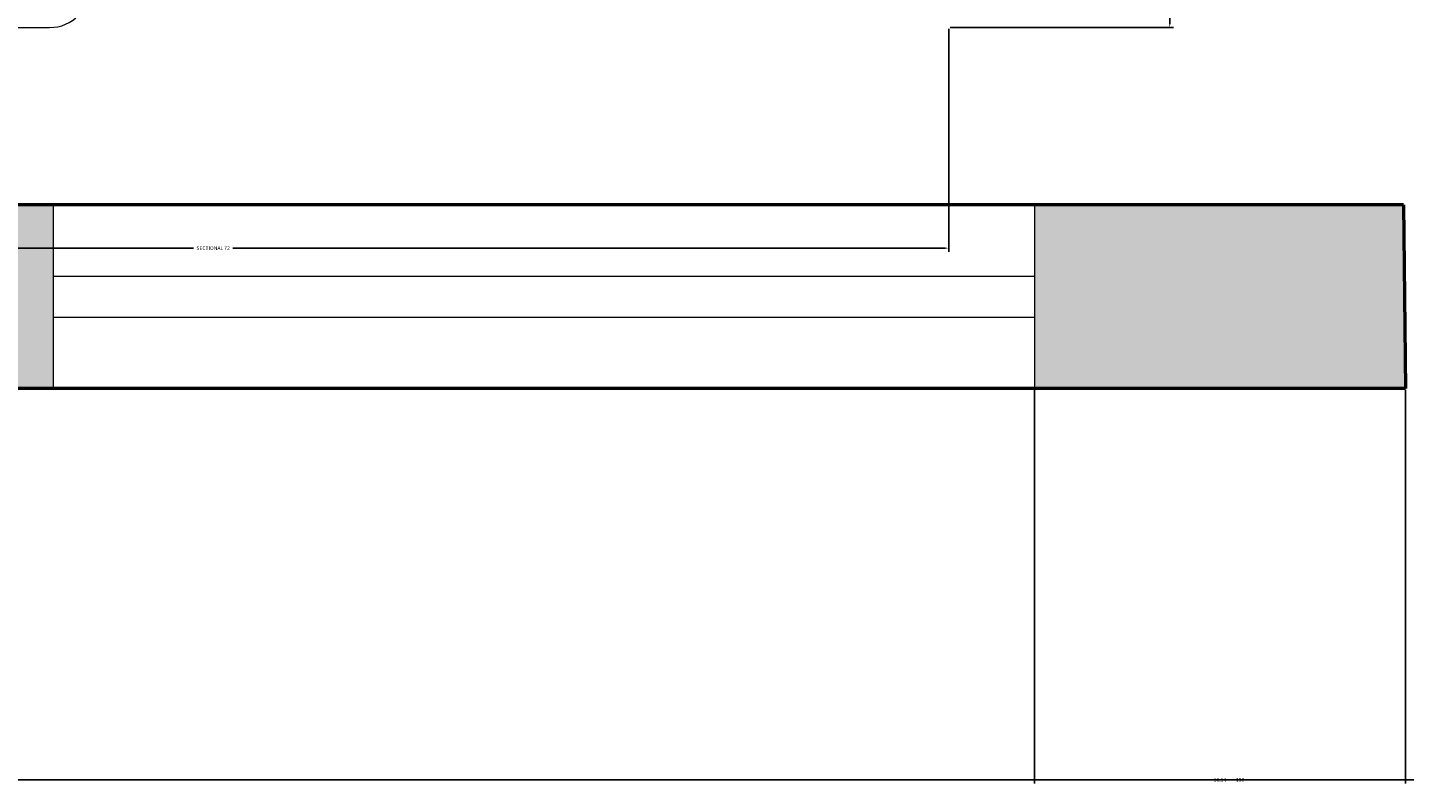
# Model space of a CAD drawing. Units: inches. Extents: x 2307 to 2544, y 2171 to 2540.
# Tile 2 of 52: x 2366 to 2434, y 2171 to 2208. Entities that reach past the tile are written whole.
import ezdxf

# ---------------------------------------------------------------- set-up
doc = ezdxf.new("R2010")
doc.units = ezdxf.units.IN
for name, color, linetype, lineweight in [('A-ANNO-DIMS', 2, 'Continuous', 18), ('A-FURN', 8, 'Continuous', 18), ('A-GLAZ', 4, 'Continuous', 18), ('A-WALL', 7, 'Continuous', 50)]:
    doc.layers.add(name, color=color, linetype=linetype, lineweight=lineweight)
doc.layers.add('A-WALL-PATT', color=18, linetype='Continuous', lineweight=13, true_color=0x000000)
doc.styles.get("Standard").update_dxf_attribs({"font": 'arial.ttf'})
doc.dimstyles.get("Standard").update_dxf_attribs({"dimtxt": 0.18, "dimasz": 0.18, "dimexe": 0.18, "dimexo": 0.0625, "dimgap": 0.09, "dimtad": 0, "dimtih": 1, "dimtoh": 1, "dimdec": 4, "dimzin": 0, "dimdsep": 46, "dimtxsty": 'Standard', "dimcen": 0.09, "dimadec": 0, "dimazin": 0, "dimtfac": 1, "dimtdec": 4, "dimtofl": 0, "dimtmove": 0, "dimatfit": 3, "dimfxl": 1, "dimtolj": 1, "dimtzin": 0, "dimarcsym": 0})

# ---------------------------------------------------------------- blocks, each defined once
blk = doc.blocks.new('sofa')
blk.add_line((-19, -66), (7, -66))
blk.add_arc((7, -64), 2, 270, 0)
blk = doc.blocks.new('WIN-48IN')
for p, q in [((0, 5.5), (48, 5.5)), ((0, 3.5), (48, 3.5))]:
    blk.add_line(p, q)
for points in [[(0, 0), (0, 9)], [(48, 9), (48, 0)]]:
    blk.add_lwpolyline(points)
blk = doc.blocks.new('*D34')
at = {"layer": 'A-ANNO-DIMS', "color": 0, "lineweight": -2, "transparency": 16777216}
for p, q in [((2339.456, 2208.123), (2339.456, 2197.206)), ((2411.456, 2208.123), (2411.456, 2197.206)), ((2339.636, 2197.386), (2374.491, 2197.386)), ((2411.276, 2197.386), (2376.421, 2197.386))]:
    blk.add_line(p, q, dxfattribs=at)
at = {"layer": 'A-ANNO-DIMS', "color": 0, "transparency": 16777216}
for points in [[(2339.636, 2197.416), (2339.636, 2197.356), (2339.456, 2197.386)], [(2411.276, 2197.416), (2411.276, 2197.356), (2411.456, 2197.386)]]:
    blk.add_solid(points, dxfattribs=at)
at = {"layer": 'Defpoints', "color": 0, "transparency": 16777216}
for p in [(2339.456, 2208.186), (2411.456, 2208.186), (2411.456, 2197.386)]:
    blk.add_point(p, dxfattribs=at)
at = {"layer": 'A-ANNO-DIMS', "color": 0, "transparency": 16777216, "insert": (2375.456, 2197.386), "char_height": 0.18, "attachment_point": 5}
blk.add_mtext('\\A1;SECTIONAL 72', dxfattribs=at)
blk = doc.blocks.new('*D35')
at = {"layer": 'A-ANNO-DIMS', "color": 0, "lineweight": -2, "transparency": 16777216}
for p, q in [((2411.518, 2280.186), (2422.436, 2280.186)), ((2422.256, 2280.006), (2422.256, 2244.366)), ((2422.256, 2208.366), (2422.256, 2244.005)), ((2411.518, 2208.186), (2422.436, 2208.186))]:
    blk.add_line(p, q, dxfattribs=at)
at = {"layer": 'A-ANNO-DIMS', "color": 0, "transparency": 16777216}
for points in [[(2422.226, 2280.006), (2422.286, 2280.006), (2422.256, 2280.186)], [(2422.226, 2208.366), (2422.286, 2208.366), (2422.256, 2208.186)]]:
    blk.add_solid(points, dxfattribs=at)
at = {"layer": 'Defpoints', "color": 0, "transparency": 16777216}
for p in [(2411.456, 2280.186), (2422.256, 2280.186), (2411.456, 2208.186)]:
    blk.add_point(p, dxfattribs=at)
at = {"layer": 'A-ANNO-DIMS', "color": 0, "transparency": 16777216, "insert": (2422.256, 2244.186), "char_height": 0.18, "attachment_point": 5}
blk.add_mtext('\\A1;72', dxfattribs=at)
blk = doc.blocks.new('*D36')
at = {"layer": 'A-ANNO-DIMS', "color": 0, "lineweight": -2, "transparency": 16777216}
for p, q in [((2326.696, 2190.447), (2326.696, 2171.18)), ((2524.696, 2190.447), (2524.696, 2171.18)), ((2326.876, 2171.36), (2425.415, 2171.36)), ((2524.516, 2171.36), (2425.976, 2171.36))]:
    blk.add_line(p, q, dxfattribs=at)
at = {"layer": 'A-ANNO-DIMS', "color": 0, "transparency": 16777216}
for points in [[(2326.876, 2171.39), (2326.876, 2171.33), (2326.696, 2171.36)], [(2524.516, 2171.39), (2524.516, 2171.33), (2524.696, 2171.36)]]:
    blk.add_solid(points, dxfattribs=at)
at = {"layer": 'Defpoints', "color": 0, "transparency": 16777216}
for p in [(2326.696, 2190.51), (2524.696, 2190.51), (2524.696, 2171.36)]:
    blk.add_point(p, dxfattribs=at)
at = {"layer": 'A-ANNO-DIMS', "color": 0, "transparency": 16777216, "insert": (2425.696, 2171.36), "char_height": 0.18, "attachment_point": 5}
blk.add_mtext('\\A1;198', dxfattribs=at)
blk = doc.blocks.new('*D38')
at = {"layer": 'A-ANNO-DIMS', "color": 0, "lineweight": -2, "transparency": 16777216}
for p, q in [((2415.642, 2190.447), (2415.642, 2171.18)), ((2433.783, 2190.447), (2433.783, 2171.18)), ((2415.822, 2171.36), (2424.328, 2171.36)), ((2433.603, 2171.36), (2425.098, 2171.36))]:
    blk.add_line(p, q, dxfattribs=at)
at = {"layer": 'A-ANNO-DIMS', "color": 0, "transparency": 16777216}
for points in [[(2415.822, 2171.39), (2415.822, 2171.33), (2415.642, 2171.36)], [(2433.603, 2171.39), (2433.603, 2171.33), (2433.783, 2171.36)]]:
    blk.add_solid(points, dxfattribs=at)
at = {"layer": 'Defpoints', "color": 0, "transparency": 16777216}
for p in [(2415.642, 2190.51), (2433.783, 2190.51), (2433.783, 2171.36)]:
    blk.add_point(p, dxfattribs=at)
at = {"layer": 'A-ANNO-DIMS', "color": 0, "transparency": 16777216, "insert": (2424.713, 2171.36), "char_height": 0.18, "attachment_point": 5}
blk.add_mtext('\\A1;18.14', dxfattribs=at)

msp = doc.modelspace()

# ---------------------------------------------------------------- hatches: boundary and pattern name
at = {"layer": 'A-WALL-PATT'}
h = msp.add_hatch(color=256, dxfattribs=at)
h.dxf.hatch_style = 1
h.paths.add_polyline_path([(2433.6935, 2199.5096), (2415.6423, 2199.5096), (2415.6423, 2190.5096), (2433.7832, 2190.5096)], flags=17)
h.paths.add_polyline_path([(2367.6423, 2199.5096), (2335.6958, 2199.5096), (2335.6958, 2307.3983), (2326.6958, 2307.3983), (2326.6958, 2190.5096), (2367.6423, 2190.5096)])
h.paths.add_polyline_path([(2524.6958, 2520.5096), (2496.7832, 2520.5096), (2496.7832, 2515.5149), (2472.7832, 2515.5149), (2472.7832, 2520.5096), (2415.4028, 2520.5096), (2415.4028, 2511.5096), (2451.6958, 2511.5096), (2451.6958, 2439.5096), (2451.6958, 2391.5096), (2445.6958, 2391.5096), (2445.6958, 2387.5096), (2455.6958, 2387.5096), (2455.6958, 2435.5096), (2461.6958, 2435.5096), (2461.6958, 2439.5096), (2455.6958, 2439.5096), (2455.6958, 2511.5096), (2515.6958, 2511.5096), (2515.6958, 2439.5096), (2491.6958, 2439.5096), (2491.6958, 2435.5096), (2515.6958, 2435.5096), (2515.6958, 2319.5096), (2451.6958, 2319.5096), (2451.6958, 2281.5096), (2481.6958, 2281.5096), (2481.6958, 2225.5096), (2485.6958, 2225.5096), (2485.6958, 2285.5096), (2455.6958, 2285.5096), (2455.6958, 2315.5096), (2515.6958, 2315.5096), (2515.6958, 2199.5096), (2469.6952, 2199.5096), (2469.785, 2190.5096), (2524.6958, 2190.5096)])

# ---------------------------------------------------------------- linework, layer by layer
at = {"layer": 'A-WALL'}
for q in [(2335.6958, 2199.5096), (2335.6958, 2199.5096), (2433.7832, 2190.5096)]:
    msp.add_line((2433.6935, 2199.5096), q, dxfattribs=at)
msp.add_lwpolyline([(2433.7832, 2190.5096), (2326.6958, 2190.5096), (2326.6958, 2520.5096), (2524.6958, 2520.5096), (2524.6958, 2190.5096), (2469.785, 2190.5096)], dxfattribs=at)

# ---------------------------------------------------------------- block references
at = {"layer": 'A-FURN'}
msp.add_blockref('sofa', (2360.4557, 2274.1858), dxfattribs=at)
at = {"layer": 'A-GLAZ'}
msp.add_blockref('WIN-48IN', (2367.642, 2190.51), dxfattribs=at)

# ---------------------------------------------------------------- dimensions: what is measured, and where the dimension line sits
at = {"layer": 'A-ANNO-DIMS'}
dim = msp.add_linear_dim(base=(2422.2557, 2280.1858), p1=(2411.4557, 2208.1858), p2=(2411.4557, 2280.1858), angle=90, dimstyle='Standard', override={"dimdec": 0, "dimlfac": 1, "dimrnd": 0, "dimzin": 0, "dimdsep": 46, "dimlunit": 2}, dxfattribs=at)
dim.commit()
dim.dimension.update_dxf_attribs({"geometry": '*D35', "text_midpoint": (2422.2557, 2244.1858)})
dim = msp.add_linear_dim(base=(2411.4557, 2197.3858), p1=(2339.4557, 2208.1858), p2=(2411.4557, 2208.1858), text='SECTIONAL <>', dimstyle='Standard', override={"dimdec": 0, "dimlfac": 1, "dimrnd": 0, "dimzin": 0, "dimdsep": 46, "dimlunit": 2}, dxfattribs=at)
dim.commit()
dim.dimension.update_dxf_attribs({"geometry": '*D34', "text_midpoint": (2375.4557, 2197.3858)})
for base, p1, p2, override, picture, middle in [((2524.6958, 2171.3596), (2326.6958, 2190.5096), (2524.6958, 2190.5096), {"dimdec": 0, "dimlfac": 1, "dimrnd": 0, "dimzin": 0, "dimdsep": 46, "dimlunit": 2}, '*D36', (2425.6958, 2171.3596)), ((2433.7832, 2171.3596), (2415.6423, 2190.5096), (2433.7832, 2190.5096), {"dimdec": 2, "dimlfac": 1, "dimrnd": 0, "dimzin": 0, "dimdsep": 46, "dimlunit": 2}, '*D38', (2424.7128, 2171.3596))]:
    dim = msp.add_linear_dim(base=base, p1=p1, p2=p2, dimstyle='Standard', override=override, dxfattribs=at)
    dim.commit()
    dim.dimension.update_dxf_attribs({"geometry": picture, "text_midpoint": middle})

doc.saveas('drawing.dxf')
